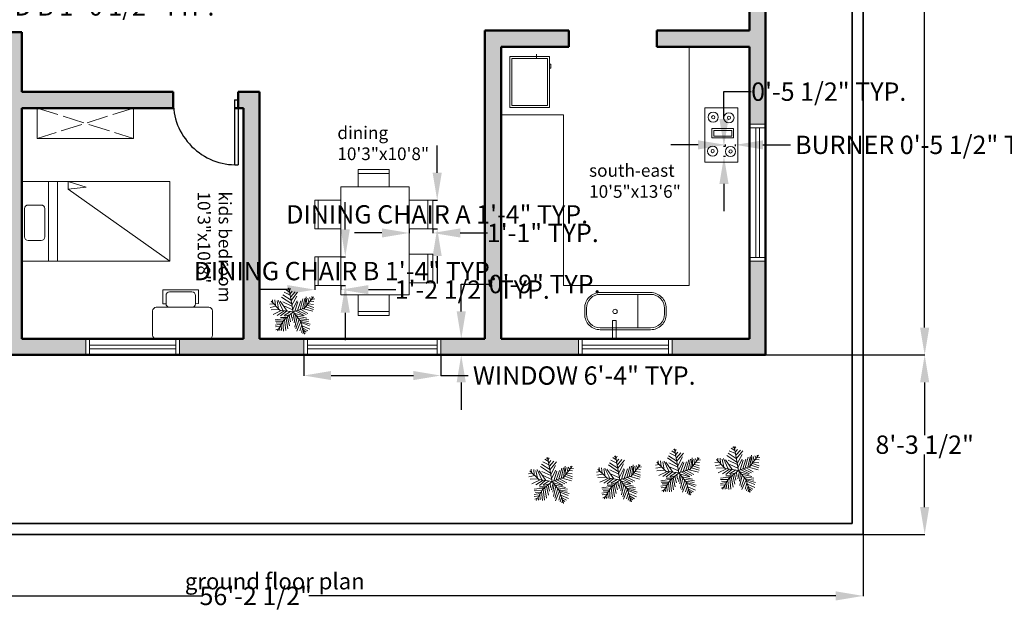
# Model space of a CAD drawing. Units: inches. Extents: x -2 to 7298, y -2 to 4583.
# Tile 2 of 6: x 6252 to 6799, y 3545 to 3880. Entities that reach past the tile are written whole.
import ezdxf

# ---------------------------------------------------------------- set-up
doc = ezdxf.new("R2010")
doc.units = ezdxf.units.IN
doc.header["$MEASUREMENT"] = 0
doc.linetypes.add('ACAD_ISO02W100', pattern=[15, 12, -3])
for name, color, linetype, lineweight in [('A-ANNO-DIMS', 2, 'Continuous', 18), ('A-ANNO-TEXT', 7, 'Continuous', 25), ('A-AREA-IDEN', 7, 'Continuous', 18), ('A-DOOR', 4, 'Continuous', 25), ('A-EQPM', 9, 'Continuous', 18), ('A-FLOR-CASE', 30, 'Continuous', 18), ('A-FLOR-CASE-HIDN', 30, 'ACAD_ISO02W100', 13), ('A-FLOR-FIXT', 9, 'Continuous', 18), ('A-FURN', 8, 'Continuous', 18), ('A-GLAZ', 4, 'Continuous', 18), ('A-WALL', 7, 'Continuous', 50), ('A-WALL-PATT', 18, 'Continuous', 13), ('C-PROP', 7, 'Continuous', 35), ('L-PLNT', 3, 'Continuous', 13)]:
    doc.layers.add(name, color=color, linetype=linetype, lineweight=lineweight)
doc.styles.get("Standard").update_dxf_attribs({"font": 'arial.ttf'})
doc.dimstyles.get("Standard").update_dxf_attribs({"dimtxt": 10.18, "dimasz": 15.18, "dimexe": 0.18, "dimexo": 0.0625, "dimgap": 0.09, "dimtad": 0, "dimtih": 1, "dimtoh": 1, "dimdec": 0, "dimzin": 0, "dimdsep": 46, "dimlunit": 3, "dimtxsty": 'Standard', "dimcen": 0.09, "dimadec": 0, "dimazin": 0, "dimtfac": 1, "dimtdec": 0, "dimtofl": 0, "dimtmove": 0, "dimatfit": 3, "dimfxl": 1, "dimtolj": 1, "dimtzin": 0, "dimarcsym": 0})

# ---------------------------------------------------------------- blocks, each defined once
blk = doc.blocks.new('*U11')
for p, q in [((-8.737, 47.138), (-17.069, 52.711)), ((-10.186, 53.64), (-13.084, 55.962)), ((0, 0), (-10.5, 57)), ((-9.099, 51.782), (-6.563, 55.962)), ((-7.65, 43.423), (-2.578, 49.46)), ((-5.839, 35.992), (4.667, 48.067)), ((-31.5, 4.5), (-52.5, 25.5)), ((-48.585, 21.131), (-49.309, 29.026)), ((-43.513, 28.561), (-42.427, 15.558)), ((-38.442, 26.239), (-34.819, 7.663)), ((-35.544, 28.097), (-24.314, 3.947)), ((-14.533, 2.09), (-30.834, 25.31)), ((-3.665, 19.273), (-27.574, 35.527)), ((-5.114, 28.097), (-24.676, 40.636)), ((-24.314, 23.917), (-2.941, 13.7)), ((-7.288, 39.707), (-21.778, 46.673)), ((-5.114, 27.632), (10.463, 46.673)), ((-2.941, 16.486), (8.652, 37.85)), ((-1.129, 6.734), (9.014, 26.704)), ((3.942, 1.625), (11.187, 24.381)), ((10.101, 3.483), (17.708, 26.239)), ((16.259, 5.805), (23.142, 31.348)), ((22.055, 7.198), (27.489, 32.277)), ((27, 9), (48, 36)), ((27.127, 9.056), (31.112, 35.992)), ((31.836, 30.883), (32.561, 16.486)), ((35.096, 32.741), (37.27, 22.524)), ((38.719, 34.134), (41.979, 28.561)), ((40.53, 25.775), (48.862, 24.846)), ((43.791, 29.954), (51.036, 30.883)), ((44.153, 36.456), (45.239, 32.741)), ((-47.498, 19.737), (-55.83, 18.344)), ((-40.615, 13.7), (-55.105, 10.913)), ((-33.37, 6.269), (-52.207, 5.34)), ((-28.299, 3.483), (-47.86, -5.805)), ((-21.416, 3.018), (-38.079, -8.128)), ((0, 0), (-31.5, 4.5)), ((-15.982, 2.09), (-30.11, -9.521)), ((0, 0), (-22.5, -19.5)), ((-6.563, 1.161), (-21.416, -8.128)), ((-20.691, 13.7), (-1.129, 4.876)), ((0, 0), (27, 9)), ((0, 0), (18, -22.5)), ((6.478, 1.625), (26.04, -8.592)), ((11.187, 3.483), (30.749, -5.805)), ((18.07, 5.805), (35.096, -3.483)), ((24.229, 7.663), (46.688, 1.625)), ((29.662, 12.307), (48.137, 6.269)), ((33.285, 16.486), (48.862, 10.913)), ((36.183, 19.737), (48.137, 17.88)), ((-17.431, -15.094), (-42.789, -18.809)), ((-24.314, -21.596), (-42.427, -22.06)), ((-22.5, -19.5), (-37.5, -45)), ((-15.257, -12.772), (-30.11, -12.772)), ((-20.691, -18.345), (-17.793, -44.352)), ((-6.563, -5.805), (-19.967, -9.985)), ((-17.069, -15.094), (-12.721, -40.172)), ((-13.446, -11.378), (-8.737, -32.741)), ((-9.461, -8.592), (-6.201, -23.453)), ((-4.752, -3.483), (-3.665, -14.629)), ((2.493, -3.019), (-1.491, -20.202)), ((1.769, -2.555), (24.229, -9.521)), ((5.029, -6.27), (2.131, -25.775)), ((9.014, -11.378), (3.58, -35.992)), ((14.085, -16.951), (6.478, -40.172)), ((7.565, -9.056), (32.198, -14.629)), ((18.07, -22.524), (8.289, -45.745)), ((12.274, -15.094), (36.907, -18.809)), ((16.259, -19.738), (36.183, -22.989)), ((18, -22.5), (27, -52.5)), ((18.433, -22.524), (40.53, -29.026)), ((-28.299, -29.026), (-42.789, -31.348)), ((-30.834, -34.135), (-42.427, -35.528)), ((-34.457, -39.708), (-40.978, -42.494)), ((-26.849, -26.24), (-40.253, -25.775)), ((-32.646, -36.921), (-31.921, -44.352)), ((-29.023, -30.884), (-27.936, -43.887)), ((-25.038, -23.918), (-22.865, -45.281)), ((20.244, -30.419), (15.897, -44.816)), ((19.157, -25.311), (38.719, -33.206)), ((22.78, -37.85), (19.519, -48.532)), ((21.331, -32.741), (39.081, -40.636)), ((22.78, -38.314), (34.372, -44.816)), ((24.591, -45.745), (23.142, -50.854)), ((24.591, -43.423), (30.749, -47.603)), ((26.764, -49.925), (28.213, -50.854))]:
    blk.add_line(p, q)
blk = doc.blocks.new('WINDOW-72IN')
for p, q in [((-2, 4.5), (-2, -4.5)), ((0, 4.5), (0, -4.5)), ((0, 1), (72, 1)), ((72, 4.5), (72, -4.5)), ((74, 4.5), (74, -4.5)), ((0, -1), (72, -1))]:
    blk.add_line(p, q)
blk = doc.blocks.new('WINDOW-48IN')
for p, q in [((-2, 4.5), (-2, -4.5)), ((0, 4.5), (0, -4.5)), ((0, 1), (48, 1)), ((48, 4.5), (48, -4.5)), ((50, 4.5), (50, -4.5)), ((0, -1), (48, -1))]:
    blk.add_line(p, q)
blk = doc.blocks.new('DOOR-SWING-36IN')
for p, q in [((0, 0), (0, 36)), ((2, 0), (2, 36)), ((2, 0), (0, 0))]:
    blk.add_line(p, q)
blk.add_arc((1, 1), 35.01, 358.3634, 91.6366)
blk = doc.blocks.new('CHAIR-DINING-A')
for p, q in [((0, 15.87), (13.15, 15.87)), ((10.36, 15.87), (10.36, 0)), ((13.15, 15.87), (13.15, 0)), ((13.15, 0), (0, 0))]:
    blk.add_line(p, q)
blk = doc.blocks.new('CHAIR-DINING-B')
for p, q in [((14.57, 15.87), (0, 15.87)), ((0, 15.87), (0, 0)), ((1.95, 15.87), (1.95, 0)), ((0, 0), (14.57, 0))]:
    blk.add_line(p, q)
blk = doc.blocks.new('RANGE-BURNER')
for radius in [2.82, 0.902]:
    blk.add_circle((0, 0), radius)
blk = doc.blocks.new('*D37')
at = {"layer": 'A-ANNO-DIMS', "color": 0, "lineweight": -2, "transparency": 16777216}
for p, q in [((6410.08, 3693.84), (6410.08, 3682.32)), ((6486.08, 3693.84), (6486.08, 3682.32)), ((6425.26, 3682.5), (6470.9, 3682.5)), ((6486.08, 3682.5), (6501.26, 3682.5))]:
    blk.add_line(p, q, dxfattribs=at)
at = {"layer": 'A-ANNO-DIMS', "color": 0, "transparency": 16777216}
for points in [[(6425.26, 3685.03), (6425.26, 3679.97), (6410.08, 3682.5)], [(6470.9, 3685.03), (6470.9, 3679.97), (6486.08, 3682.5)]]:
    blk.add_solid(points, dxfattribs=at)
at = {"layer": 'Defpoints', "color": 0, "transparency": 16777216}
for p in [(6410.08, 3693.9), (6486.08, 3693.9), (6486.08, 3682.5)]:
    blk.add_point(p, dxfattribs=at)
at = {"layer": 'A-ANNO-DIMS', "color": 0, "transparency": 16777216, "insert": (6565.76, 3682.5), "char_height": 10.18, "attachment_point": 5}
blk.add_mtext('\\A1;WINDOW 6\'-4" TYP.', dxfattribs=at)
blk = doc.blocks.new('*D38')
at = {"layer": 'A-ANNO-DIMS', "color": 0, "lineweight": -2, "transparency": 16777216}
for p, q in [((6497.48, 3718.08), (6497.48, 3733.26)), ((6497.48, 3733.26), (6512.66, 3733.26)), ((6486.14, 3702.9), (6497.66, 3702.9)), ((6486.14, 3693.9), (6497.66, 3693.9)), ((6497.48, 3678.72), (6497.48, 3663.54))]:
    blk.add_line(p, q, dxfattribs=at)
at = {"layer": 'A-ANNO-DIMS', "color": 0, "transparency": 16777216}
for points in [[(6494.95, 3718.08), (6500.01, 3718.08), (6497.48, 3702.9)], [(6494.95, 3678.72), (6500.01, 3678.72), (6497.48, 3693.9)]]:
    blk.add_solid(points, dxfattribs=at)
at = {"layer": 'Defpoints', "color": 0, "transparency": 16777216}
for p in [(6486.08, 3702.9), (6497.48, 3702.9), (6486.08, 3693.9)]:
    blk.add_point(p, dxfattribs=at)
at = {"layer": 'A-ANNO-DIMS', "color": 0, "transparency": 16777216, "insert": (6543.77, 3733.26), "char_height": 10.18, "attachment_point": 5}
blk.add_mtext('\\A1;0\'-9" TYP.', dxfattribs=at)
blk = doc.blocks.new('*D45')
at = {"layer": 'A-ANNO-DIMS', "color": 0, "lineweight": -2, "transparency": 16777216}
for p, q in [((6628.99, 3810.47), (6613.81, 3810.47)), ((6644.17, 3809.69), (6644.17, 3810.65)), ((6649.81, 3809.69), (6649.81, 3810.65)), ((6664.99, 3810.47), (6680.17, 3810.47))]:
    blk.add_line(p, q, dxfattribs=at)
at = {"layer": 'A-ANNO-DIMS', "color": 0, "transparency": 16777216}
for points in [[(6628.99, 3813), (6628.99, 3807.94), (6644.17, 3810.47)], [(6664.99, 3813), (6664.99, 3807.94), (6649.81, 3810.47)]]:
    blk.add_solid(points, dxfattribs=at)
at = {"layer": 'Defpoints', "color": 0, "transparency": 16777216}
for p in [(6649.81, 3810.47), (6644.17, 3809.63), (6649.81, 3809.63)]:
    blk.add_point(p, dxfattribs=at)
at = {"layer": 'A-ANNO-DIMS', "color": 0, "transparency": 16777216, "insert": (6754.93, 3810.47), "char_height": 10.18, "attachment_point": 5}
blk.add_mtext('\\A1;BURNER 0\'-5 1/2" TYP.', dxfattribs=at)
blk = doc.blocks.new('*D46')
at = {"layer": 'A-ANNO-DIMS', "color": 0, "lineweight": -2, "transparency": 16777216}
for p, q in [((6643.32, 3824.81), (6643.32, 3839.99)), ((6643.32, 3839.99), (6658.5, 3839.99)), ((6644.1, 3809.63), (6643.14, 3809.63)), ((6644.1, 3803.98), (6643.14, 3803.98)), ((6643.32, 3788.8), (6643.32, 3773.62))]:
    blk.add_line(p, q, dxfattribs=at)
at = {"layer": 'A-ANNO-DIMS', "color": 0, "transparency": 16777216}
for points in [[(6640.79, 3824.81), (6645.85, 3824.81), (6643.32, 3809.63)], [(6640.79, 3788.8), (6645.85, 3788.8), (6643.32, 3803.98)]]:
    blk.add_solid(points, dxfattribs=at)
at = {"layer": 'Defpoints', "color": 0, "transparency": 16777216}
for p in [(6643.32, 3809.63), (6644.17, 3809.63), (6644.17, 3803.98)]:
    blk.add_point(p, dxfattribs=at)
at = {"layer": 'A-ANNO-DIMS', "color": 0, "transparency": 16777216, "insert": (6701.48, 3839.99), "char_height": 10.18, "attachment_point": 5}
blk.add_mtext('\\A1;0\'-5 1/2" TYP.', dxfattribs=at)
blk = doc.blocks.new('*D47')
at = {"layer": 'A-ANNO-DIMS', "color": 0, "lineweight": -2, "transparency": 16777216}
for p, q in [((6484.13, 3795.02), (6484.13, 3810.2)), ((6481.81, 3779.84), (6484.31, 3779.84)), ((6481.81, 3763.97), (6484.31, 3763.97)), ((6484.13, 3748.79), (6484.13, 3733.61))]:
    blk.add_line(p, q, dxfattribs=at)
at = {"layer": 'A-ANNO-DIMS', "color": 0, "transparency": 16777216}
for points in [[(6481.6, 3795.02), (6486.66, 3795.02), (6484.13, 3779.84)], [(6481.6, 3748.79), (6486.66, 3748.79), (6484.13, 3763.97)]]:
    blk.add_solid(points, dxfattribs=at)
at = {"layer": 'Defpoints', "color": 0, "transparency": 16777216}
for p in [(6481.75, 3779.84), (6484.13, 3779.84), (6481.75, 3763.97)]:
    blk.add_point(p, dxfattribs=at)
at = {"layer": 'A-ANNO-DIMS', "color": 0, "transparency": 16777216, "insert": (6484.13, 3771.91), "char_height": 10.18, "attachment_point": 5}
blk.add_mtext('\\A1;DINING CHAIR A 1\'-4" TYP.', dxfattribs=at)
blk = doc.blocks.new('*D48')
at = {"layer": 'A-ANNO-DIMS', "color": 0, "lineweight": -2, "transparency": 16777216}
for p, q in [((6453.42, 3761.59), (6438.24, 3761.59)), ((6468.6, 3763.91), (6468.6, 3761.41)), ((6481.75, 3763.91), (6481.75, 3761.41)), ((6496.93, 3761.59), (6512.11, 3761.59))]:
    blk.add_line(p, q, dxfattribs=at)
at = {"layer": 'A-ANNO-DIMS', "color": 0, "transparency": 16777216}
for points in [[(6453.42, 3764.12), (6453.42, 3759.06), (6468.6, 3761.59)], [(6496.93, 3764.12), (6496.93, 3759.06), (6481.75, 3761.59)]]:
    blk.add_solid(points, dxfattribs=at)
at = {"layer": 'Defpoints', "color": 0, "transparency": 16777216}
for p in [(6468.6, 3763.97), (6481.75, 3763.97), (6481.75, 3761.59)]:
    blk.add_point(p, dxfattribs=at)
at = {"layer": 'A-ANNO-DIMS', "color": 0, "transparency": 16777216, "insert": (6542.75, 3761.59), "char_height": 10.18, "attachment_point": 5}
blk.add_mtext('\\A1;1\'-1" TYP.', dxfattribs=at)
blk = doc.blocks.new('*D49')
at = {"layer": 'A-ANNO-DIMS', "color": 0, "lineweight": -2, "transparency": 16777216}
for p, q in [((6433.11, 3763.58), (6433.11, 3778.76)), ((6430.79, 3748.4), (6433.29, 3748.4)), ((6430.79, 3732.53), (6433.29, 3732.53)), ((6433.11, 3717.35), (6433.11, 3702.17))]:
    blk.add_line(p, q, dxfattribs=at)
at = {"layer": 'A-ANNO-DIMS', "color": 0, "transparency": 16777216}
for points in [[(6430.58, 3763.58), (6435.64, 3763.58), (6433.11, 3748.4)], [(6430.58, 3717.35), (6435.64, 3717.35), (6433.11, 3732.53)]]:
    blk.add_solid(points, dxfattribs=at)
at = {"layer": 'Defpoints', "color": 0, "transparency": 16777216}
for p in [(6430.73, 3748.4), (6433.11, 3748.4), (6430.73, 3732.53)]:
    blk.add_point(p, dxfattribs=at)
at = {"layer": 'A-ANNO-DIMS', "color": 0, "transparency": 16777216, "insert": (6433.11, 3740.46), "char_height": 10.18, "attachment_point": 5}
blk.add_mtext('\\A1;DINING CHAIR B 1\'-4" TYP.', dxfattribs=at)
blk = doc.blocks.new('*D50')
at = {"layer": 'A-ANNO-DIMS', "color": 0, "lineweight": -2, "transparency": 16777216}
for p, q in [((6400.98, 3730.15), (6385.8, 3730.15)), ((6416.16, 3732.47), (6416.16, 3729.97)), ((6430.73, 3732.47), (6430.73, 3729.97)), ((6445.91, 3730.15), (6461.09, 3730.15))]:
    blk.add_line(p, q, dxfattribs=at)
at = {"layer": 'A-ANNO-DIMS', "color": 0, "transparency": 16777216}
for points in [[(6400.98, 3732.68), (6400.98, 3727.62), (6416.16, 3730.15)], [(6445.91, 3732.68), (6445.91, 3727.62), (6430.73, 3730.15)]]:
    blk.add_solid(points, dxfattribs=at)
at = {"layer": 'Defpoints', "color": 0, "transparency": 16777216}
for p in [(6416.16, 3732.53), (6430.73, 3732.53), (6430.73, 3730.15)]:
    blk.add_point(p, dxfattribs=at)
at = {"layer": 'A-ANNO-DIMS', "color": 0, "transparency": 16777216, "insert": (6503.58, 3730.15), "char_height": 10.18, "attachment_point": 5}
blk.add_mtext('\\A1;1\'-2 1/2" TYP.', dxfattribs=at)
blk = doc.blocks.new('*D55')
at = {"layer": 'A-ANNO-DIMS', "color": 0, "lineweight": -2, "transparency": 16777216}
for p, q in [((6110.57, 3887.28), (6095.39, 3887.28)), ((6125.75, 3889.11), (6125.75, 3887.1)), ((6138.34, 3889.11), (6138.34, 3887.1)), ((6153.52, 3887.28), (6168.7, 3887.28))]:
    blk.add_line(p, q, dxfattribs=at)
at = {"layer": 'A-ANNO-DIMS', "color": 0, "transparency": 16777216}
for points in [[(6110.57, 3889.81), (6110.57, 3884.75), (6125.75, 3887.28)], [(6153.52, 3889.81), (6153.52, 3884.75), (6138.34, 3887.28)]]:
    blk.add_solid(points, dxfattribs=at)
at = {"layer": 'Defpoints', "color": 0, "transparency": 16777216}
for p in [(6125.75, 3889.17), (6138.34, 3889.17), (6138.34, 3887.28)]:
    blk.add_point(p, dxfattribs=at)
at = {"layer": 'A-ANNO-DIMS', "color": 0, "transparency": 16777216, "insert": (6266.35, 3887.28), "char_height": 10.18, "attachment_point": 5}
blk.add_mtext('\\A1;NIGHTSTAND B 1\'-0 1/2" TYP.', dxfattribs=at)
blk = doc.blocks.new('*D61')
at = {"layer": 'A-ANNO-DIMS', "color": 0, "lineweight": -2, "transparency": 16777216}
for p, q in [((6046.17, 3594.33), (6046.17, 3560.06)), ((6720.58, 3594.33), (6720.58, 3560.06)), ((6061.35, 3560.24), (6353.94, 3560.24)), ((6705.4, 3560.24), (6412.81, 3560.24))]:
    blk.add_line(p, q, dxfattribs=at)
at = {"layer": 'A-ANNO-DIMS', "color": 0, "transparency": 16777216}
for points in [[(6061.35, 3562.77), (6061.35, 3557.71), (6046.17, 3560.24)], [(6705.4, 3562.77), (6705.4, 3557.71), (6720.58, 3560.24)]]:
    blk.add_solid(points, dxfattribs=at)
at = {"layer": 'Defpoints', "color": 0, "transparency": 16777216}
for p in [(6046.17, 3594.39), (6720.58, 3594.39), (6720.58, 3560.24)]:
    blk.add_point(p, dxfattribs=at)
at = {"layer": 'A-ANNO-DIMS', "color": 0, "transparency": 16777216, "insert": (6383.37, 3560.24), "char_height": 10.18, "attachment_point": 5}
blk.add_mtext('\\A1;56\'-2 1/2"', dxfattribs=at)
blk = doc.blocks.new('*D65')
at = {"layer": 'A-ANNO-DIMS', "color": 0, "lineweight": -2, "transparency": 16777216}
for p, q in [((6720.64, 4097.9), (6754.91, 4097.9)), ((6754.73, 4082.72), (6754.73, 3901.2)), ((6754.73, 3709.08), (6754.73, 3890.61)), ((6666.54, 3693.9), (6754.91, 3693.9))]:
    blk.add_line(p, q, dxfattribs=at)
at = {"layer": 'A-ANNO-DIMS', "color": 0, "transparency": 16777216}
for points in [[(6752.2, 4082.72), (6757.26, 4082.72), (6754.73, 4097.9)], [(6752.2, 3709.08), (6757.26, 3709.08), (6754.73, 3693.9)]]:
    blk.add_solid(points, dxfattribs=at)
at = {"layer": 'Defpoints', "color": 0, "transparency": 16777216}
for p in [(6720.58, 4097.9), (6754.73, 4097.9), (6666.47, 3693.9)]:
    blk.add_point(p, dxfattribs=at)
at = {"layer": 'A-ANNO-DIMS', "color": 0, "transparency": 16777216, "insert": (6754.73, 3895.9), "char_height": 10.18, "attachment_point": 5}
blk.add_mtext('\\A1;33\'-8"', dxfattribs=at)
blk = doc.blocks.new('*D67')
at = {"layer": 'A-ANNO-DIMS', "color": 0, "lineweight": -2, "transparency": 16777216}
for p, q in [((6666.54, 3693.9), (6754.91, 3693.9)), ((6754.73, 3678.72), (6754.73, 3649.5)), ((6754.73, 3609.57), (6754.73, 3638.79)), ((6720.64, 3594.39), (6754.91, 3594.39))]:
    blk.add_line(p, q, dxfattribs=at)
at = {"layer": 'A-ANNO-DIMS', "color": 0, "transparency": 16777216}
for points in [[(6752.2, 3678.72), (6757.26, 3678.72), (6754.73, 3693.9)], [(6752.2, 3609.57), (6757.26, 3609.57), (6754.73, 3594.39)]]:
    blk.add_solid(points, dxfattribs=at)
at = {"layer": 'Defpoints', "color": 0, "transparency": 16777216}
for p in [(6666.47, 3693.9), (6720.58, 3594.39), (6754.73, 3594.39)]:
    blk.add_point(p, dxfattribs=at)
at = {"layer": 'A-ANNO-DIMS', "color": 0, "transparency": 16777216, "insert": (6754.73, 3644.15), "char_height": 10.18, "attachment_point": 5}
blk.add_mtext('\\A1;8\'-3 1/2"', dxfattribs=at)
blk = doc.blocks.new('*D68')
at = {"layer": 'A-ANNO-DIMS', "color": 0, "lineweight": -2, "transparency": 16777216}
for p, q in [((6666.47, 3693.97), (6666.47, 4134.81)), ((6681.65, 4134.63), (6705.4, 4134.63)), ((6720.58, 3594.45), (6720.58, 4134.81)), ((6720.58, 4134.63), (6735.76, 4134.63))]:
    blk.add_line(p, q, dxfattribs=at)
at = {"layer": 'A-ANNO-DIMS', "color": 0, "transparency": 16777216}
for points in [[(6681.65, 4137.16), (6681.65, 4132.1), (6666.47, 4134.63)], [(6705.4, 4137.16), (6705.4, 4132.1), (6720.58, 4134.63)]]:
    blk.add_solid(points, dxfattribs=at)
at = {"layer": 'Defpoints', "color": 0, "transparency": 16777216}
for p in [(6720.58, 4134.63), (6666.47, 3693.9), (6720.58, 3594.39)]:
    blk.add_point(p, dxfattribs=at)
at = {"layer": 'A-ANNO-DIMS', "color": 0, "transparency": 16777216, "insert": (6749.58, 4134.63), "char_height": 10.18, "attachment_point": 5}
blk.add_mtext('\\A1;4\'-6"', dxfattribs=at)

msp = doc.modelspace()

# ---------------------------------------------------------------- hatches: boundary and pattern name
at = {"layer": 'A-WALL-PATT'}
h = msp.add_hatch(color=256, dxfattribs=at)
h.dxf.hatch_style = 1
h.paths.add_polyline_path([(6253.58, 3872.9), (6244.58, 3872.9), (6244.58, 3869.9), (6121.58, 3869.9), (6121.58, 3906.9), (6112.58, 3906.9), (6112.58, 3860.9), (6244.58, 3860.9), (6244.58, 3693.9), (6289.08, 3693.9), (6289.08, 3702.9), (6253.58, 3702.9), (6253.58, 3830.9), (6337.58, 3830.9), (6337.58, 3833.4, -0.014283), (6337.58, 3835.4), (6337.58, 3839.9), (6253.58, 3839.9)])
h.paths.add_polyline_path([(6385.58, 3839.9), (6373.58, 3839.9), (6373.58, 3830.9), (6376.58, 3830.9), (6376.58, 3702.9), (6341.08, 3702.9), (6341.08, 3693.9), (6410.08, 3693.9), (6410.08, 3702.9), (6385.58, 3702.9)])
h.paths.add_polyline_path([(6519.58, 3864.9), (6557.19, 3864.9), (6557.19, 3873.9), (6510.58, 3873.9), (6510.58, 3839.9), (6510.58, 3702.9), (6486.08, 3702.9), (6486.08, 3693.9), (6562.53, 3693.9), (6562.53, 3702.9), (6519.58, 3702.9)])
h.paths.add_polyline_path([(6666.47, 3745.9), (6657.47, 3745.9), (6657.47, 3702.9), (6614.53, 3702.9), (6614.53, 3693.9), (6666.47, 3693.9)])
h.paths.add_polyline_path([(6666.47, 3926.97), (6661.97, 3926.97, -0.014283), (6659.97, 3926.97), (6657.47, 3926.97), (6657.47, 3873.9), (6606.04, 3873.9), (6606.04, 3864.9), (6657.47, 3864.9), (6657.47, 3821.9), (6666.47, 3821.9)])
h.paths.add_polyline_path([(6720.58, 4097.9), (6547.84, 4097.9), (6547.84, 4088.9), (6606.58, 4088.9), (6606.58, 3997.9, 0.414214), (6608.58, 3995.9), (6618.58, 3995.9), (6618.58, 4004.9), (6615.58, 4004.9), (6615.58, 4088.9), (6711.58, 4088.9), (6711.58, 4060.9), (6720.58, 4060.9)])
h.paths.add_polyline_path([(6720.58, 4032.9), (6711.58, 4032.9), (6711.58, 4004.9), (6654.58, 4004.9), (6654.58, 4002.4, -0.014283), (6654.58, 4000.4), (6654.58, 3995.9), (6711.58, 3995.9), (6720.58, 3995.9)], flags=17)
h.paths.add_polyline_path([(6471.84, 4097.9), (6233.45, 4097.9), (6233.45, 4088.9), (6244.58, 4088.9), (6244.58, 4004.9), (6244.58, 3995.9), (6244.58, 3908.9), (6247.08, 3908.9, -0.014283), (6249.08, 3908.9), (6253.58, 3908.9), (6253.58, 3995.9), (6253.58, 4088.9), (6392.58, 4088.9), (6392.58, 4004.9), (6392.58, 3995.9), (6392.58, 3894.9), (6401.58, 3894.9), (6401.58, 3995.9), (6401.58, 4004.9), (6401.58, 4088.9), (6471.84, 4088.9)])
h.paths.add_polyline_path([(6205.45, 4097.9), (6112.58, 4097.9), (6112.58, 4060.9), (6121.58, 4060.9), (6121.58, 4088.9), (6186.64, 4088.9), (6186.64, 4034.49), (6189.14, 4034.49, -0.021729), (6191.14, 4034.49), (6195.64, 4034.49), (6195.64, 4088.9), (6202.58, 4088.9), (6205.45, 4088.9)])
h.paths.add_polyline_path([(6121.58, 3995.9), (6217.58, 3995.9), (6217.58, 4000.4, -0.021729), (6217.58, 4002.4), (6217.58, 4004.9), (6195.64, 4004.9), (6195.64, 4010.49), (6186.64, 4010.49), (6186.64, 4004.9), (6121.58, 4004.9), (6121.58, 4032.9), (6112.58, 4032.9), (6112.58, 3958.9), (6121.58, 3958.9)])

# ---------------------------------------------------------------- linework, layer by layer
at = {"layer": 'A-EQPM'}
for points in [[(6546.4, 3859.44), (6546.4, 3859.44), (6546.4, 3831.27), (6546.4, 3831.27), (6524.54, 3831.27), (6524.54, 3831.27), (6524.54, 3859.44), (6524.54, 3859.44)], [(6539.33, 3860.77), (6539.33, 3860.77), (6539.33, 3858.55), (6539.33, 3858.55), (6539.33, 3858.55), (6539.33, 3858.55), (6539.33, 3860.77), (6539.33, 3860.77)], [(6545.4, 3858.44), (6545.4, 3832.27), (6525.54, 3832.27), (6525.54, 3858.44)], [(6546.4, 3855.3), (6546.4, 3855.3), (6546.4, 3853.02), (6546.4, 3853.02), (6547.3, 3853.02), (6547.3, 3853.02), (6547.3, 3855.3), (6547.3, 3855.3)], [(6632.61, 3831.09), (6632.61, 3831.09), (6651.08, 3831.09), (6651.08, 3831.09), (6651.08, 3800.86), (6651.08, 3800.86), (6632.61, 3800.86), (6632.61, 3800.86)], [(6636.62, 3819.49), (6636.62, 3819.49), (6648.63, 3819.49), (6648.63, 3819.49), (6648.63, 3814.33), (6648.63, 3814.33), (6636.62, 3814.33), (6636.62, 3814.33)], [(6637.62, 3818.49), (6647.63, 3818.49), (6647.63, 3815.33), (6637.62, 3815.33)]]:
    msp.add_lwpolyline(points, close=True, dxfattribs=at)
at = {"layer": 'A-FLOR-CASE'}
for p, q in [((6623.93, 3732.44), (6623.93, 3864.9)), ((6262.16, 3830.9), (6262.16, 3813.94)), ((6315.49, 3813.94), (6315.49, 3830.9)), ((6519.58, 3827.16), (6554.16, 3827.16)), ((6554.16, 3827.16), (6554.16, 3732.44)), ((6262.16, 3813.94), (6315.49, 3813.94)), ((6554.16, 3732.44), (6623.93, 3732.44))]:
    msp.add_line(p, q, dxfattribs=at)
at = {"layer": 'A-FLOR-CASE-HIDN'}
for p, q in [((6262.16, 3830.9), (6315.49, 3813.94)), ((6315.49, 3830.9), (6262.16, 3813.94))]:
    msp.add_line(p, q, dxfattribs=at)
at = {"layer": 'A-FLOR-FIXT'}
msp.add_line((6595.59, 3727.54), (6595.59, 3708.92), dxfattribs=at)
for points in [[(6566, 3719.92, -0.414214), (6574.62, 3728.54), (6602.63, 3728.54, -0.414214), (6611.25, 3719.92), (6611.25, 3716.54, -0.414214), (6602.63, 3707.92), (6574.62, 3707.92, -0.414214), (6566, 3716.54)], [(6567, 3719.92, -0.414214), (6574.62, 3727.54), (6602.63, 3727.54, -0.414214), (6610.25, 3719.92), (6610.25, 3716.54, -0.414214), (6602.63, 3708.92), (6574.62, 3708.92, -0.414214), (6567, 3716.54)]]:
    msp.add_lwpolyline(points, format="xyb", close=True, dxfattribs=at)
msp.add_lwpolyline([(6581.41, 3702.9), (6581.41, 3702.9), (6583.56, 3702.9), (6583.56, 3702.9), (6583.56, 3713.05), (6583.56, 3713.05), (6581.41, 3713.05), (6581.41, 3713.05)], close=True, dxfattribs=at)
msp.add_circle((6582.87, 3718.03), 1.2, dxfattribs=at)
at = {"layer": 'A-FURN'}
for p, q in [((6440.22, 3787.18), (6440.22, 3796.87)), ((6440.22, 3796.87), (6457.4, 3796.87)), ((6440.22, 3794.62), (6457.4, 3794.62)), ((6457.4, 3796.87), (6457.4, 3787.18)), ((6268.41, 3790.1), (6268.41, 3745.9)), ((6273.43, 3790.1), (6273.43, 3745.9)), ((6279.3, 3785.93), (6279.3, 3790.1)), ((6279.3, 3790.1), (6289.33, 3786.91)), ((6289.33, 3786.91), (6279.3, 3785.93)), ((6279.3, 3785.93), (6335.68, 3745.9)), ((6331.81, 3722.36), (6331.81, 3730.05)), ((6331.81, 3730.05), (6351.61, 3730.05)), ((6351.61, 3730.05), (6351.61, 3722.45)), ((6333.59, 3722.36), (6331.81, 3722.36)), ((6351.61, 3722.45), (6350.01, 3722.36)), ((6440.22, 3718.03), (6457.4, 3718.03))]:
    msp.add_line(p, q, dxfattribs=at)
for points in [[(6253.58, 3790.1), (6253.58, 3790.1), (6335.68, 3790.1), (6335.68, 3790.1), (6335.68, 3745.9), (6335.68, 3745.9), (6253.58, 3745.9), (6253.58, 3745.9)], [(6430.73, 3787.18), (6430.73, 3787.18), (6468.6, 3787.18), (6468.6, 3787.18), (6468.6, 3727.34), (6468.6, 3727.34), (6430.73, 3727.34), (6430.73, 3727.34)], [(6440.22, 3727.34), (6440.22, 3727.34), (6457.4, 3727.34), (6457.4, 3727.34), (6457.4, 3715.81), (6457.4, 3715.81), (6440.22, 3715.81), (6440.22, 3715.81)]]:
    msp.add_lwpolyline(points, close=True, dxfattribs=at)
for points in [[(6255.07, 3775.08, -0.414214), (6257.07, 3777.08), (6264.28, 3777.08, -0.414214), (6266.28, 3775.08), (6266.28, 3759.45, -0.414214), (6264.28, 3757.45), (6257.07, 3757.45, -0.414214), (6255.07, 3759.45)], [(6333.59, 3722.36, 0.414214), (6335.59, 3720.36), (6348.01, 3720.36, 0.414214), (6350.01, 3722.36), (6350.01, 3726.89, 0.414214), (6348.01, 3728.89), (6335.59, 3728.89, 0.414214), (6333.59, 3726.89)], [(6359.41, 3704.9, -0.414214), (6357.41, 3702.9), (6328.17, 3702.9, -0.414214), (6326.17, 3704.9), (6326.17, 3718.36, -0.414214), (6328.17, 3720.36), (6357.41, 3720.36, -0.414214), (6359.41, 3718.36)]]:
    msp.add_lwpolyline(points, format="xyb", close=True, dxfattribs=at)
at = {"layer": 'A-WALL'}
for p, q in [((6657.47, 3927.13), (6657.47, 3873.9)), ((6666.47, 3926.97), (6666.47, 3693.9)), ((6244.58, 3872.9), (6253.58, 3872.9)), ((6253.58, 3839.9), (6253.58, 3872.9)), ((6510.58, 3839.9), (6510.58, 3873.9)), ((6557.19, 3873.9), (6510.58, 3873.9)), ((6557.19, 3873.9), (6557.19, 3864.9)), ((6657.47, 3873.9), (6606.04, 3873.9)), ((6606.04, 3864.9), (6606.04, 3873.9)), ((6519.58, 3702.9), (6519.58, 3864.9)), ((6557.19, 3864.9), (6519.58, 3864.9)), ((6657.47, 3864.9), (6606.04, 3864.9)), ((6657.47, 3864.9), (6657.47, 3702.9)), ((6337.58, 3839.9), (6253.58, 3839.9)), ((6337.58, 3830.9), (6337.58, 3839.9)), ((6385.58, 3839.9), (6373.58, 3839.9)), ((6373.58, 3830.9), (6373.58, 3839.9)), ((6385.58, 3702.9), (6385.58, 3839.9)), ((6510.58, 3702.9), (6510.58, 3839.9)), ((6253.58, 3702.9), (6253.58, 3830.9)), ((6337.74, 3830.9), (6253.58, 3830.9)), ((6376.58, 3830.9), (6371.58, 3830.9)), ((6376.58, 3702.9), (6376.58, 3830.9)), ((6376.58, 3702.9), (6253.58, 3702.9)), ((6510.58, 3702.9), (6385.58, 3702.9)), ((6657.47, 3702.9), (6519.58, 3702.9)), ((6666.47, 3693.9), (6244.58, 3693.9)), ((6666.47, 3693.9), (6385.58, 3693.9))]:
    msp.add_line(p, q, dxfattribs=at)
at = {"layer": 'C-PROP'}
for p, q in [((6714.58, 3995.9), (6714.58, 3600.39)), ((6720.58, 3995.9), (6720.58, 3594.39)), ((6714.58, 3600.39), (6052.17, 3600.39)), ((6720.58, 3594.39), (6046.17, 3594.39))]:
    msp.add_line(p, q, dxfattribs=at)

# ---------------------------------------------------------------- block references
at = {"layer": 'A-DOOR', "rotation": 180}
msp.add_blockref('DOOR-SWING-36IN', (6373.58, 3835.4), dxfattribs=at)
at = {"layer": 'A-EQPM'}
for p in [(6637.34, 3825.79), (6646.1, 3825.48), (6637.04, 3807), (6646.99, 3806.8)]:
    msp.add_blockref('RANGE-BURNER', p, dxfattribs=at)
at = {"layer": 'A-FURN'}
for name, p in [('CHAIR-DINING-B', (6416.16, 3763.97)), ('CHAIR-DINING-A', (6468.6, 3763.97)), ('CHAIR-DINING-A', (6468.6, 3734.02)), ('CHAIR-DINING-B', (6416.16, 3732.53))]:
    msp.add_blockref(name, p, dxfattribs=at)
at = {"layer": 'A-GLAZ'}
for name, p, rotation in [('WINDOW-72IN', (6661.97, 3819.9), 270.0000000000041), ('WINDOW-48IN', (6612.53, 3698.4), 180)]:
    msp.add_blockref(name, p, dxfattribs=dict(at, rotation=rotation))
for name, p in [('WINDOW-48IN', (6291.08, 3698.4)), ('WINDOW-72IN', (6412.08, 3698.4))]:
    msp.add_blockref(name, p, dxfattribs=at)
at = {"layer": 'L-PLNT', "xscale": 0.2336039447018575, "yscale": 0.2336039447018575, "zscale": 0.2336039447018575}
for p in [(6404.21, 3717.76), (6618.34, 3628.48), (6651.36, 3629.9), (6547.87, 3623.77), (6585.58, 3624.64)]:
    msp.add_blockref('*U11', p, dxfattribs=at)

# ---------------------------------------------------------------- texts
at = {"layer": 'A-ANNO-TEXT', "insert": (6344.07, 3572.88), "char_height": 9, "attachment_point": 1}
msp.add_mtext_dynamic_manual_height_columns('ground floor plan', width=436.0251, gutter_width=1, heights=[0], dxfattribs=at)
at = {"layer": 'A-AREA-IDEN', "char_height": 7, "attachment_point": 1}
for s, insert in [('dining\\P10\'3"x10\'8"', (6428.71, 3820.68)), ('south-east\\P10\'5"x13\'6"', (6568.45, 3799.77))]:
    msp.add_mtext_dynamic_manual_height_columns(s, width=127.1277, gutter_width=1, heights=[0], dxfattribs=dict(at, insert=insert))
at = {"layer": 'A-AREA-IDEN', "insert": (6369.83, 3784.63), "char_height": 7, "attachment_point": 1, "rotation": 270}
msp.add_mtext_dynamic_manual_height_columns('kids bedroom\\P10\'3"x10\'8"', width=78.7387, gutter_width=1, heights=[0], dxfattribs=at)

# ---------------------------------------------------------------- dimensions: what is measured, and where the dimension line sits
at = {"layer": 'A-ANNO-DIMS'}
for base, p1, picture, middle in [((6720.58, 4134.63), (6666.47, 3693.9), '*D68', (6749.58, 4134.63)), ((6720.58, 3560.24), (6046.17, 3594.39), '*D61', (6383.37, 3560.24))]:
    dim = msp.add_linear_dim(base=base, p1=p1, p2=(6720.58, 3594.39), dimstyle='Standard', override={"dimdec": 1, "dimlfac": 1, "dimrnd": 0, "dimzin": 1, "dimdsep": 46, "dimlunit": 4, "dimfrac": 2}, dxfattribs=at)
    dim.commit()
    dim.dimension.update_dxf_attribs({"geometry": picture, "text_midpoint": middle})
for base, p2, picture, middle in [((6754.73, 4097.9), (6720.58, 4097.9), '*D65', (6754.73, 3895.9)), ((6754.73, 3594.39), (6720.58, 3594.39), '*D67', (6754.73, 3644.15))]:
    dim = msp.add_linear_dim(base=base, p1=(6666.47, 3693.9), p2=p2, angle=90, dimstyle='Standard', override={"dimdec": 1, "dimlfac": 1, "dimrnd": 0, "dimzin": 1, "dimdsep": 46, "dimlunit": 4, "dimfrac": 2}, dxfattribs=at)
    dim.commit()
    dim.dimension.update_dxf_attribs({"geometry": picture, "text_midpoint": middle})
for base, p1, p2, text, picture, middle in [((6138.34, 3887.28), (6125.75, 3889.17), (6138.34, 3889.17), 'NIGHTSTAND B <> TYP.', '*D55', (6266.35, 3887.28)), ((6649.81, 3810.47), (6644.17, 3809.63), (6649.81, 3809.63), 'BURNER <> TYP.', '*D45', (6754.93, 3810.47)), ((6481.7518, 3761.5946), (6468.5997, 3763.9748), (6481.7518, 3763.9748), '<> TYP.', '*D48', (6542.7487, 3761.5946)), ((6430.73, 3730.15), (6416.16, 3732.53), (6430.73, 3732.53), '<> TYP.', '*D50', (6503.58, 3730.15)), ((6486.08, 3682.5), (6410.08, 3693.9), (6486.08, 3693.9), 'WINDOW <> TYP.', '*D37', (6565.76, 3682.5))]:
    dim = msp.add_linear_dim(base=base, p1=p1, p2=p2, text=text, dimstyle='Standard', override={"dimdec": 1, "dimlfac": 1, "dimrnd": 0, "dimzin": 1, "dimdsep": 46, "dimlunit": 4, "dimfrac": 2}, dxfattribs=at)
    dim.commit()
    dim.dimension.update_dxf_attribs({"geometry": picture, "text_midpoint": middle})
for base, p1, p2, text, picture, middle in [((6643.3189, 3809.6272), (6644.1662, 3803.9785), (6644.1662, 3809.6272), '<> TYP.', '*D46', (6701.4755, 3839.9872)), ((6484.13, 3779.84), (6481.75, 3763.97), (6481.75, 3779.84), 'DINING CHAIR A <> TYP.', '*D47', (6484.13, 3771.91)), ((6433.11, 3748.4), (6430.73, 3732.53), (6430.73, 3748.4), 'DINING CHAIR B <> TYP.', '*D49', (6433.11, 3740.46)), ((6497.48, 3702.9), (6486.08, 3693.9), (6486.08, 3702.9), '<> TYP.', '*D38', (6543.77, 3733.26))]:
    dim = msp.add_linear_dim(base=base, p1=p1, p2=p2, angle=90, text=text, dimstyle='Standard', override={"dimdec": 1, "dimlfac": 1, "dimrnd": 0, "dimzin": 1, "dimdsep": 46, "dimlunit": 4, "dimfrac": 2}, dxfattribs=at)
    dim.commit()
    dim.dimension.update_dxf_attribs({"geometry": picture, "text_midpoint": middle})

doc.saveas('drawing.dxf')
